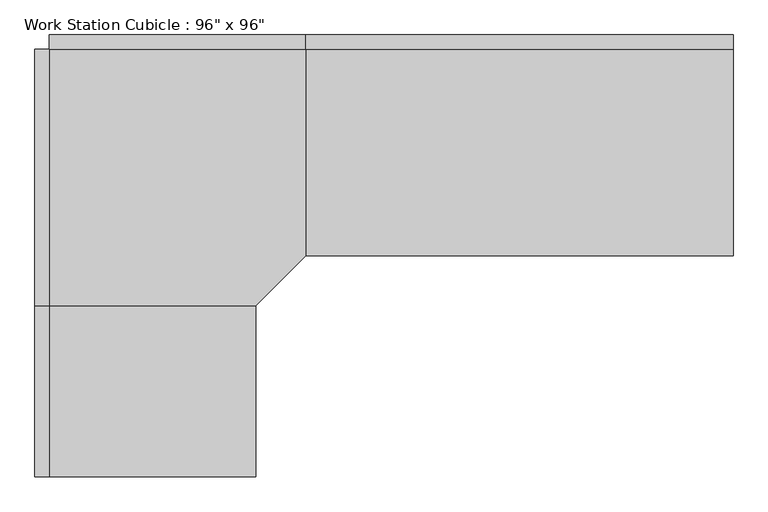
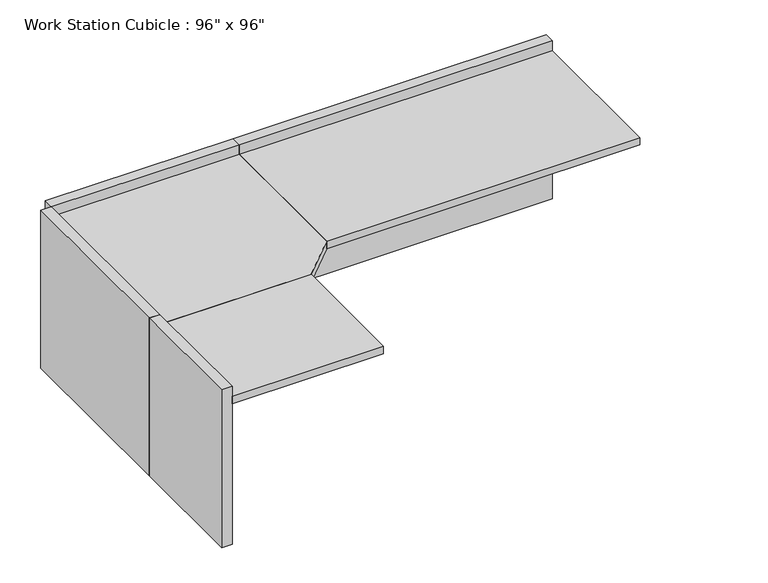
"""IFC4 building model written with IfcOpenShell, lengths in millimetres: furniture geometry."""

from ifc_helpers import new_model, si_unit, frame, origin, origin_with_axes, place, context, project, spatial, polyline, outline, extrude, source, transform, mapped, element, save


def furniture_be658349(model_context):
    return source(origin(), model_context, "Body", "SweptSolid", [
        extrude(outline(polyline([(-80.9317522, -545.8230076), (833.4682478, -545.8230076), (833.4682478, -1282.4230076), (655.6682478, -1460.2230076), (-80.9317522, -1460.2230076), (-80.9317522, -545.8230076)])), frame((0.0, 0.0, 723.9), z_axis=(0.0, 0.0, 1.0), x_axis=(1.0, 0.0, 0.0)), (0.0, 0.0, 1.0), 38.1),
        extrude(outline(polyline([(655.6682478, -2069.8230076), (-80.9317522, -2069.8230076), (-80.9317522, -1460.2230076), (655.6682478, -1460.2230076), (655.6682478, -2069.8230076)])), frame((0.0, 0.0, 723.9), z_axis=(0.0, 0.0, 1.0), x_axis=(1.0, 0.0, 0.0)), (0.0, 0.0, 1.0), 38.1),
        extrude(outline(polyline([(2357.4682478, -1282.4230076), (833.4682478, -1282.4230076), (833.4682478, -545.8230076), (2357.4682478, -545.8230076), (2357.4682478, -1282.4230076)])), frame((0.0, 0.0, 723.9), z_axis=(0.0, 0.0, 1.0), x_axis=(1.0, 0.0, 0.0)), (0.0, 0.0, 1.0), 38.1),
        extrude(outline(polyline([(2357.4682478, -545.8230076), (833.4682478, -545.8230076), (833.4682478, -495.0230076), (2357.4682478, -495.0230076), (2357.4682478, -545.8230076)])), origin_with_axes(), (0.0, 0.0, 1.0), 812.8),
        extrude(outline(polyline([(833.4682478, -545.8230076), (-80.9317522, -545.8230076), (-80.9317522, -495.0230076), (833.4682478, -495.0230076), (833.4682478, -545.8230076)])), origin_with_axes(), (0.0, 0.0, 1.0), 812.8),
        extrude(outline(polyline([(-80.9317522, -1460.2230076), (-131.7317522, -1460.2230076), (-131.7317522, -545.8230076), (-80.9317522, -545.8230076), (-80.9317522, -1460.2230076)])), origin_with_axes(), (0.0, 0.0, 1.0), 812.8),
        extrude(outline(polyline([(-80.9317522, -2069.8230076), (-131.7317522, -2069.8230076), (-131.7317522, -1460.2230076), (-80.9317522, -1460.2230076), (-80.9317522, -2069.8230076)])), origin_with_axes(), (0.0, 0.0, 1.0), 812.8),
    ])


if __name__ == "__main__":
    model = new_model("IFC4")
    model_context = context("Model", 3, world=origin())
    ifc_project = project(units=[si_unit("LENGTHUNIT", "METRE", prefix="MILLI")], contexts=[model_context])
    site = spatial("IfcSite", under=ifc_project)
    building = spatial("IfcBuilding", under=site)
    placement = place(None, origin())
    furniture_shape = furniture_be658349(model_context)
    element("IfcFurniture", 1, ObjectType="Work Station Cubicle : 96\" x 96\"", at=placement, inside=building, context=model_context, shape_type="MappedRepresentation", body=[
        mapped(furniture_shape, transform((0.0, 0.0, 0.0), x_axis=(1.0, 0.0, 0.0), y_axis=(0.0, 1.0, 0.0), z_axis=(0.0, 0.0, 1.0))),
    ])
    save(model, "model.ifc")

# Revit data of these elements
# Type "Work Station Cubicle : 96\" x 96\""
#   Assembly Code = "E2020"
#   Desktop Height = 2' - 6"
#   Desktop1 Width = 2' - 5"
#   Desktop2 Width = 2' - 5"
#   Panel Height = 2' - 8"
#   Panel1 Length = 2' - 0"
#   Panel2 Length = 5' - 0"
#   Cube Panel Material = Textile - Light Gray
#   Work Top Material = Laminate, Ivory, Matte
#   Default Elevation = 0
# Element 1 (IfcFurniture, "Work Station Cubicle : 96\" x 96\"")
#   Materials on its faces: "Textile - Light Gray", "Laminate, Ivory, Matte"
# Materials
#   "Textile - Light Gray": class "Fabric", colour RGB 204 204 204, transparency 0
#   "Laminate, Ivory, Matte": class "Plastic", colour RGB 247 247 239, transparency 0, Description = "Plastic Laminate - Ivory, Matte", Cost = 0
